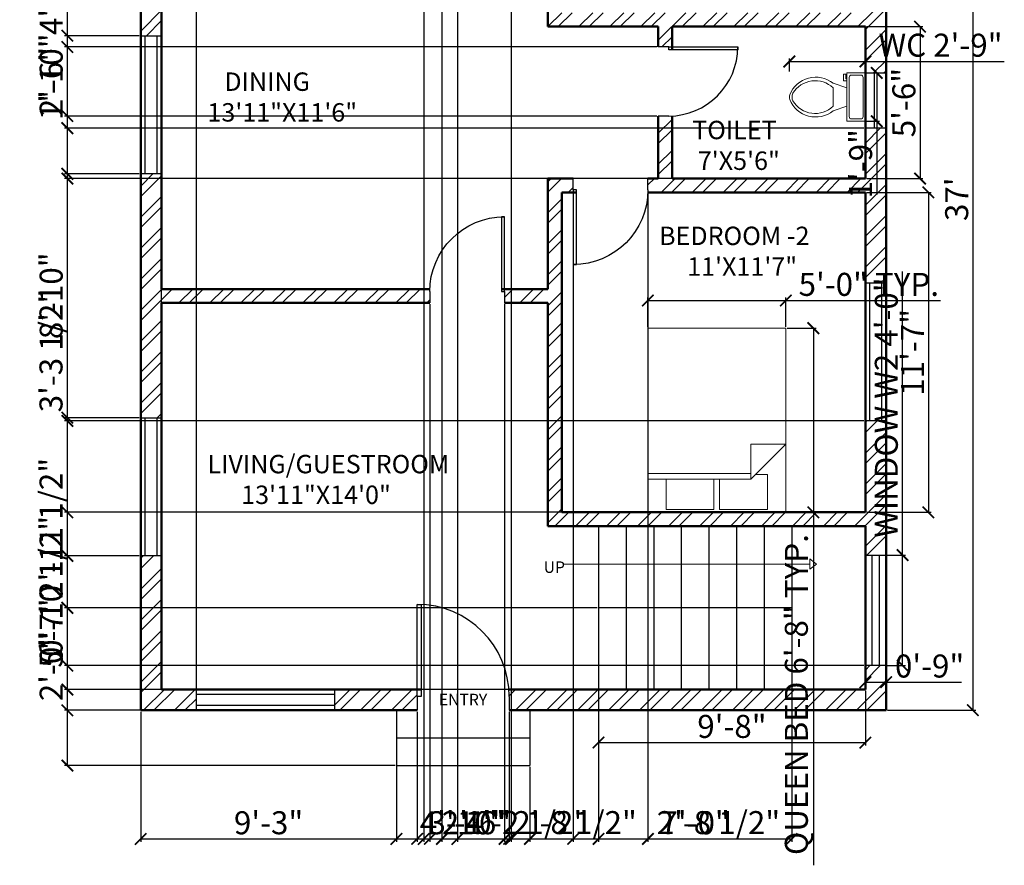
# Model space of a CAD drawing. Units: inches. Extents: x 9 to 670, y -4 to 628.
# Tile 1 of 2: x 9 to 437, y -4 to 363. Entities that reach past the tile are written whole.
import ezdxf

# ---------------------------------------------------------------- set-up
doc = ezdxf.new("R2010")
doc.units = ezdxf.units.IN
for name, color, linetype, lineweight in [('A-ANNO-SYMB', 1, 'Continuous', 18), ('A-AREA-IDEN', 1, 'Continuous', 25), ('A-FLOR-FIXT', 2, 'Continuous', 18), ('A-FLOR-STRS', 7, 'Continuous', 25), ('A-FURN', 2, 'Continuous', 18), ('A-WALL-PATT', 9, 'Continuous', 13), ('DIM', 3, 'Continuous', 18), ('DOORS', 4, 'Continuous', 25), ('TEXT', 1, 'Continuous', 25), ('VENTILATOR', 11, 'Continuous', 25), ('WALLS', 6, 'Continuous', 50), ('WINDOWS', 20, 'Continuous', 25)]:
    doc.layers.add(name, color=color, linetype=linetype, lineweight=lineweight)
doc.styles.get("Standard").update_dxf_attribs({"font": 'arial.ttf'})
doc.dimstyles.new('ISO-25', dxfattribs={"dimtxt": 10, "dimasz": 5, "dimexe": 1.25, "dimexo": 0.625, "dimtad": 1, "dimlunit": 4, "dimtxsty": 'Standard', "dimblk": 'ARCHTICK', "dimcen": 2.5, "dimadec": 0, "dimazin": 0, "dimtfac": 1, "dimtmove": 0, "dimatfit": 3, "dimfxl": 1, "dimarcsym": 0})

# ---------------------------------------------------------------- blocks, each defined once
blk = doc.blocks.new('Toilet - top')
for p, q in [((9.5, -6), (9.5, -2)), ((-10, -8.5), (-8, -8.5)), ((-10, -9.5), (-10, -8.5)), ((-8, -8.5), (-8, -8)), ((-7, -8), (-7, -9.5)), ((-4, -8), (-6, -14)), ((4, -8), (6, -14)), ((-7, -9.5), (-10, -9.5)), ((4, -14), (-4, -14))]:
    blk.add_line(p, q)
blk.add_lwpolyline([(10.5, -8), (10.5, 0), (-10.5, 0), (-10.5, -8)], close=True)
for points in [[(-9.5, -2), (-9.5, -6)], [(8.5, -1), (-8.5, -1)], [(-8.5, -7), (8.5, -7)]]:
    blk.add_lwpolyline(points)
for centre, radius, start, end in [((-8.62, -1.88), 0.884, 81.8699, 188.1301), ((8.62, -1.88), 0.884, 351.8699, 98.1301), ((-8.62, -6.12), 0.884, 171.8699, 278.1301), ((8.62, -6.12), 0.884, 261.8699, 8.1301), ((3.52, -21.58), 12.17, 141.4691, 247.9714), ((4.2, -21.82), 11.33, 136.3677, 238.9468), ((-3.52, -21.58), 12.17, 292.0284, 38.5307), ((-4.2, -21.82), 11.33, 301.053, 43.6321), ((0, -27.88), 4, 245.7318, 294.2682), ((0, -29), 4, 254.8605, 285.1395)]:
    blk.add_arc(centre, radius, start, end)
blk = doc.blocks.new('Bed - Queen')
for p, q in [((0, -80.00003), (0, 0)), ((0, 0), (59.99999, 0)), ((59.99999, 0), (59.99999, -80.00003)), ((7.99999, -1.2), (28.79998, -1.2)), ((7.99999, -14.4), (7.99999, -1.2)), ((28.79998, -1.2), (28.79998, -14.4)), ((31.19999, -1.2), (51.99999, -1.2)), ((31.19999, -14.4), (31.19999, -1.2)), ((51.99999, -1.2), (51.99999, -16.4)), ((0, -14.4), (44.8, -14.4)), ((44.8, -16.8), (0, -16.8)), ((59.99999, -29.6), (44.8, -14.4)), ((44.8, -14.4), (44.8, -29.6)), ((51.99999, -16.4), (46.79936, -16.4)), ((44.8, -29.6), (59.99999, -29.6)), ((59.99999, -80.00003), (0, -80.00003))]:
    blk.add_line(p, q)
blk = doc.blocks.new('*U8')
for p, q in [((0, 0), (0, -6)), ((40, 0), (40, -6))]:
    blk.add_line(p, q)
blk.add_lwpolyline([(0, 0), (0, 40), (1.75, 40), (1.75, 0)], close=True)
blk.add_arc((0, 0), 40, 0, 90)
blk = doc.blocks.new('W2')
at = {"layer": 'WINDOWS'}
for p, q in [((1126.75, 2245.25), (1135.75, 2245.25)), ((1126.75, 2197.25), (1126.75, 2245.25)), ((1129.75, 2197.25), (1129.75, 2245.25)), ((1132.75, 2245.25), (1132.75, 2197.25)), ((1135.75, 2245.25), (1135.75, 2197.25)), ((1135.75, 2197.25), (1126.75, 2197.25))]:
    blk.add_line(p, q, dxfattribs=at)
blk = doc.blocks.new('W1')
at = {"layer": 'WINDOWS'}
for p, q in [((1078.63, 2170.04), (1087.63, 2170.04)), ((1078.63, 2110.04), (1078.63, 2170.04)), ((1080.63, 2110.04), (1080.63, 2170.04)), ((1085.63, 2170.04), (1085.63, 2110.04)), ((1087.63, 2170.04), (1087.63, 2110.04)), ((1087.63, 2110.04), (1078.63, 2110.04))]:
    blk.add_line(p, q, dxfattribs=at)
blk = doc.blocks.new('VENTILATOR')
at = {"layer": 'VENTILATOR'}
for p, q in [((1084.96, 2166.43), (1093.96, 2166.43)), ((1084.96, 2142.43), (1084.96, 2166.43)), ((1088.96, 2142.43), (1088.96, 2166.43)), ((1089.96, 2166.43), (1089.96, 2142.43)), ((1093.96, 2166.43), (1093.96, 2142.43)), ((1093.96, 2142.43), (1084.96, 2142.43))]:
    blk.add_line(p, q, dxfattribs=at)
blk = doc.blocks.new('_ArchTick')
at = {"color": 0, "linetype": 'ByBlock', "const_width": 0.15}
blk.add_lwpolyline([(-0.5, -0.5), (0.5, 0.5)], dxfattribs=at)
blk = doc.blocks.new('*D13')
at = {"layer": 'Defpoints', "color": 0, "transparency": 16777216}
for p in [(376.85, 360.12), (376.85, 294.12), (400.61, 294.12)]:
    blk.add_point(p, dxfattribs=at)
at = {"layer": 'DIM', "color": 0, "lineweight": -2, "transparency": 16777216}
for p, q in [((377.48, 360.12), (401.86, 360.12)), ((400.61, 360.12), (400.61, 294.12)), ((377.48, 294.12), (401.86, 294.12))]:
    blk.add_line(p, q, dxfattribs=at)
at = {"layer": 'DIM', "color": 0, "lineweight": -2, "transparency": 16777216, "xscale": 5, "yscale": 5, "zscale": 5}
for p, rotation in [((400.61, 360.12), 90), ((400.61, 294.12), 270)]:
    blk.add_blockref('_ArchTick', p, dxfattribs=dict(at, rotation=rotation))
at = {"layer": 'DIM', "color": 0, "transparency": 16777216, "insert": (394.88, 327.12), "char_height": 10, "attachment_point": 5, "rotation": 90}
blk.add_mtext('5\'-6"', dxfattribs=at)
blk = doc.blocks.new('*D14')
at = {"layer": 'Defpoints', "color": 0, "transparency": 16777216}
for p in [(376.85, 288.12), (376.85, 149.12), (404.24, 149.12)]:
    blk.add_point(p, dxfattribs=at)
at = {"layer": 'DIM', "color": 0, "lineweight": -2, "transparency": 16777216}
for p, q in [((377.48, 288.12), (405.49, 288.12)), ((404.24, 288.12), (404.24, 149.12)), ((377.48, 149.12), (405.49, 149.12))]:
    blk.add_line(p, q, dxfattribs=at)
at = {"layer": 'DIM', "color": 0, "lineweight": -2, "transparency": 16777216, "xscale": 5, "yscale": 5, "zscale": 5}
for p, rotation in [((404.24, 288.12), 90), ((404.24, 149.12), 270)]:
    blk.add_blockref('_ArchTick', p, dxfattribs=dict(at, rotation=rotation))
at = {"layer": 'DIM', "color": 0, "transparency": 16777216, "insert": (398.59, 218.62), "char_height": 10, "attachment_point": 5, "rotation": 90}
blk.add_mtext('11\'-7"', dxfattribs=at)
blk = doc.blocks.new('*D15')
at = {"layer": 'Defpoints', "color": 0, "transparency": 16777216}
for p in [(385.85, 507.12), (385.85, 63.12), (423.57, 63.12)]:
    blk.add_point(p, dxfattribs=at)
at = {"layer": 'DIM', "color": 0, "lineweight": -2, "transparency": 16777216}
for p, q in [((386.48, 507.12), (424.82, 507.12)), ((423.57, 507.12), (423.57, 63.12)), ((386.48, 63.12), (424.82, 63.12))]:
    blk.add_line(p, q, dxfattribs=at)
at = {"layer": 'DIM', "color": 0, "lineweight": -2, "transparency": 16777216, "xscale": 5, "yscale": 5, "zscale": 5}
for p, rotation in [((423.57, 507.12), 90), ((423.57, 63.12), 270)]:
    blk.add_blockref('_ArchTick', p, dxfattribs=dict(at, rotation=rotation))
at = {"layer": 'DIM', "color": 0, "transparency": 16777216, "insert": (417.84, 285.12), "char_height": 10, "attachment_point": 5, "rotation": 90}
blk.add_mtext("37'", dxfattribs=at)
blk = doc.blocks.new('*D20')
at = {"layer": 'Defpoints', "color": 0, "transparency": 16777216}
for p in [(260.85, 72.12), (376.85, 72.12), (376.85, 49.08)]:
    blk.add_point(p, dxfattribs=at)
at = {"layer": 'DIM', "color": 0, "lineweight": -2, "transparency": 16777216}
for p, q in [((260.85, 71.49), (260.85, 47.83)), ((376.85, 71.49), (376.85, 47.83)), ((260.85, 49.08), (376.85, 49.08))]:
    blk.add_line(p, q, dxfattribs=at)
at = {"layer": 'DIM', "color": 0, "lineweight": -2, "transparency": 16777216, "xscale": 5, "yscale": 5, "zscale": 5, "rotation": 180}
blk.add_blockref('_ArchTick', (260.85, 49.08), dxfattribs=at)
at = {"layer": 'DIM', "color": 0, "lineweight": -2, "transparency": 16777216, "xscale": 5, "yscale": 5, "zscale": 5}
blk.add_blockref('_ArchTick', (376.85, 49.08), dxfattribs=at)
at = {"layer": 'DIM', "color": 0, "transparency": 16777216, "insert": (318.85, 54.81), "char_height": 10, "attachment_point": 5}
blk.add_mtext('9\'-8"', dxfattribs=at)
blk = doc.blocks.new('*D23')
at = {"layer": 'Defpoints', "color": 0, "transparency": 16777216}
for p in [(385.85, 130.51), (393.05, 130.51), (385.85, 82.51)]:
    blk.add_point(p, dxfattribs=at)
at = {"layer": 'DIM', "color": 0, "lineweight": -2, "transparency": 16777216}
for p, q in [((393.05, 130.51), (393.05, 253.77)), ((386.48, 130.51), (394.3, 130.51)), ((393.05, 82.51), (393.05, 130.51)), ((386.48, 82.51), (394.3, 82.51))]:
    blk.add_line(p, q, dxfattribs=at)
at = {"layer": 'DIM', "color": 0, "lineweight": -2, "transparency": 16777216, "xscale": 5, "yscale": 5, "zscale": 5}
for p, rotation in [((393.05, 130.51), 90), ((393.05, 82.51), 270)]:
    blk.add_blockref('_ArchTick', p, dxfattribs=dict(at, rotation=rotation))
at = {"layer": 'DIM', "color": 0, "transparency": 16777216, "insert": (387.25, 194.64), "char_height": 10, "attachment_point": 5, "rotation": 90}
blk.add_mtext('WINDOW W2 4\'-0"', dxfattribs=at)
blk = doc.blocks.new('*D24')
at = {"layer": 'Defpoints', "color": 0, "transparency": 16777216}
for p in [(376.85, 82.51), (385.85, 82.51), (385.85, 75.31)]:
    blk.add_point(p, dxfattribs=at)
at = {"layer": 'DIM', "color": 0, "lineweight": -2, "transparency": 16777216}
for p, q in [((376.85, 81.89), (376.85, 74.06)), ((385.85, 81.89), (385.85, 74.06)), ((376.85, 75.31), (385.85, 75.31)), ((385.85, 75.31), (418.68, 75.31))]:
    blk.add_line(p, q, dxfattribs=at)
at = {"layer": 'DIM', "color": 0, "lineweight": -2, "transparency": 16777216, "xscale": 5, "yscale": 5, "zscale": 5, "rotation": 180}
blk.add_blockref('_ArchTick', (376.85, 75.31), dxfattribs=at)
at = {"layer": 'DIM', "color": 0, "lineweight": -2, "transparency": 16777216, "xscale": 5, "yscale": 5, "zscale": 5}
blk.add_blockref('_ArchTick', (385.85, 75.31), dxfattribs=at)
at = {"layer": 'DIM', "color": 0, "transparency": 16777216, "insert": (404.77, 81.04), "char_height": 10, "attachment_point": 5}
blk.add_mtext('0\'-9"', dxfattribs=at)
blk = doc.blocks.new('*D27')
at = {"layer": 'Defpoints', "color": 0, "transparency": 16777216}
for p in [(376.85, 344.96), (343.8, 340), (376.85, 340)]:
    blk.add_point(p, dxfattribs=at)
at = {"layer": 'DIM', "color": 0, "lineweight": -2, "transparency": 16777216}
for p, q in [((343.8, 340.63), (343.8, 346.21)), ((343.8, 344.96), (376.85, 344.96)), ((376.85, 340.63), (376.85, 346.21)), ((376.85, 344.96), (437.25, 344.96))]:
    blk.add_line(p, q, dxfattribs=at)
at = {"layer": 'DIM', "color": 0, "lineweight": -2, "transparency": 16777216, "xscale": 5, "yscale": 5, "zscale": 5, "rotation": 180}
blk.add_blockref('_ArchTick', (343.8, 344.96), dxfattribs=at)
at = {"layer": 'DIM', "color": 0, "lineweight": -2, "transparency": 16777216, "xscale": 5, "yscale": 5, "zscale": 5}
blk.add_blockref('_ArchTick', (376.85, 344.96), dxfattribs=at)
at = {"layer": 'DIM', "color": 0, "transparency": 16777216, "insert": (409.55, 350.75), "char_height": 10, "attachment_point": 5}
blk.add_mtext('WC 2\'-9"', dxfattribs=at)
blk = doc.blocks.new('*D28')
at = {"layer": 'Defpoints', "color": 0, "transparency": 16777216}
for p in [(376.85, 340), (376.85, 319), (381.81, 319)]:
    blk.add_point(p, dxfattribs=at)
at = {"layer": 'DIM', "color": 0, "lineweight": -2, "transparency": 16777216}
for p, q in [((377.48, 340), (383.06, 340)), ((381.81, 340), (381.81, 319)), ((377.48, 319), (383.06, 319)), ((381.81, 319), (381.81, 287.11))]:
    blk.add_line(p, q, dxfattribs=at)
at = {"layer": 'DIM', "color": 0, "lineweight": -2, "transparency": 16777216, "xscale": 5, "yscale": 5, "zscale": 5}
for p, rotation in [((381.81, 340), 90), ((381.81, 319), 270)]:
    blk.add_blockref('_ArchTick', p, dxfattribs=dict(at, rotation=rotation))
at = {"layer": 'DIM', "color": 0, "transparency": 16777216, "insert": (376.08, 300.55), "char_height": 10, "attachment_point": 5, "rotation": 90}
blk.add_mtext('1\'-9"', dxfattribs=at)
blk = doc.blocks.new('*D29')
at = {"layer": 'Defpoints', "color": 0, "transparency": 16777216}
for p in [(342.24, 229.12), (342.24, 149.12), (354.24, 149.12)]:
    blk.add_point(p, dxfattribs=at)
at = {"layer": 'DIM', "color": 0, "lineweight": -2, "transparency": 16777216}
for p, q in [((342.87, 229.12), (355.49, 229.12)), ((354.24, 229.12), (354.24, 149.12)), ((342.87, 149.12), (355.49, 149.12)), ((354.24, 149.12), (354.24, -4.23))]:
    blk.add_line(p, q, dxfattribs=at)
at = {"layer": 'DIM', "color": 0, "lineweight": -2, "transparency": 16777216, "xscale": 5, "yscale": 5, "zscale": 5}
for p, rotation in [((354.24, 229.12), 90), ((354.24, 149.12), 270)]:
    blk.add_blockref('_ArchTick', p, dxfattribs=dict(at, rotation=rotation))
at = {"layer": 'DIM', "color": 0, "transparency": 16777216, "insert": (348.14, 69.94), "char_height": 10, "attachment_point": 5, "rotation": 90}
blk.add_mtext('QUEEN BED 6\'-8" TYP.', dxfattribs=at)
blk = doc.blocks.new('*D30')
at = {"layer": 'Defpoints', "color": 0, "transparency": 16777216}
for p in [(342.24, 241.12), (282.24, 229.12), (342.24, 229.12)]:
    blk.add_point(p, dxfattribs=at)
at = {"layer": 'DIM', "color": 0, "lineweight": -2, "transparency": 16777216}
for p, q in [((282.24, 229.74), (282.24, 242.37)), ((282.24, 241.12), (342.24, 241.12)), ((342.24, 229.74), (342.24, 242.37)), ((342.24, 241.12), (409.45, 241.12))]:
    blk.add_line(p, q, dxfattribs=at)
at = {"layer": 'DIM', "color": 0, "lineweight": -2, "transparency": 16777216, "xscale": 5, "yscale": 5, "zscale": 5, "rotation": 180}
blk.add_blockref('_ArchTick', (282.24, 241.12), dxfattribs=at)
at = {"layer": 'DIM', "color": 0, "lineweight": -2, "transparency": 16777216, "xscale": 5, "yscale": 5, "zscale": 5}
blk.add_blockref('_ArchTick', (342.24, 241.12), dxfattribs=at)
at = {"layer": 'DIM', "color": 0, "transparency": 16777216, "insert": (378.35, 246.85), "char_height": 10, "attachment_point": 5}
blk.add_mtext('5\'-0" TYP.', dxfattribs=at)
blk = doc.blocks.new('*D35')
at = {"layer": 'Defpoints', "color": 0, "transparency": 16777216}
for p in [(173.01, 39.12), (231.01, 39.12), (231.01, 7.22)]:
    blk.add_point(p, dxfattribs=at)
at = {"layer": 'DIM', "color": 0, "lineweight": -2, "transparency": 16777216}
for p, q in [((173.01, 38.49), (173.01, 5.97)), ((231.01, 38.49), (231.01, 5.97)), ((173.01, 7.22), (231.01, 7.22))]:
    blk.add_line(p, q, dxfattribs=at)
at = {"layer": 'DIM', "color": 0, "lineweight": -2, "transparency": 16777216, "xscale": 5, "yscale": 5, "zscale": 5, "rotation": 180}
blk.add_blockref('_ArchTick', (173.01, 7.22), dxfattribs=at)
at = {"layer": 'DIM', "color": 0, "lineweight": -2, "transparency": 16777216, "xscale": 5, "yscale": 5, "zscale": 5}
blk.add_blockref('_ArchTick', (231.01, 7.22), dxfattribs=at)
at = {"layer": 'DIM', "color": 0, "transparency": 16777216, "insert": (202.01, 12.95), "char_height": 10, "attachment_point": 5}
blk.add_mtext('4\'-10"', dxfattribs=at)
blk = doc.blocks.new('*D36')
at = {"layer": 'Defpoints', "color": 0, "transparency": 16777216}
for p in [(29.95, 63.12), (173.01, 63.12), (173.01, 39.12)]:
    blk.add_point(p, dxfattribs=at)
at = {"layer": 'DIM', "color": 0, "lineweight": -2, "transparency": 16777216}
for p, q in [((29.95, 63.12), (29.95, 96.12)), ((172.39, 63.12), (28.7, 63.12)), ((29.95, 39.12), (29.95, 63.12)), ((172.39, 39.12), (28.7, 39.12))]:
    blk.add_line(p, q, dxfattribs=at)
at = {"layer": 'DIM', "color": 0, "lineweight": -2, "transparency": 16777216, "xscale": 5, "yscale": 5, "zscale": 5}
for p, rotation in [((29.95, 63.12), 90), ((29.95, 39.12), 270)]:
    blk.add_blockref('_ArchTick', p, dxfattribs=dict(at, rotation=rotation))
at = {"layer": 'DIM', "color": 0, "transparency": 16777216, "insert": (24.22, 82.12), "char_height": 10, "attachment_point": 5, "rotation": 90}
blk.add_mtext('2\'-0"', dxfattribs=at)
blk = doc.blocks.new('*D37')
at = {"layer": 'Defpoints', "color": 0, "transparency": 16777216}
for p in [(182.01, 63.12), (222.01, 63.12), (222.01, 7.22)]:
    blk.add_point(p, dxfattribs=at)
at = {"layer": 'DIM', "color": 0, "lineweight": -2, "transparency": 16777216}
for p, q in [((182.01, 62.49), (182.01, 5.97)), ((222.01, 62.49), (222.01, 5.97)), ((182.01, 7.22), (222.01, 7.22))]:
    blk.add_line(p, q, dxfattribs=at)
at = {"layer": 'DIM', "color": 0, "lineweight": -2, "transparency": 16777216, "xscale": 5, "yscale": 5, "zscale": 5, "rotation": 180}
blk.add_blockref('_ArchTick', (182.01, 7.22), dxfattribs=at)
at = {"layer": 'DIM', "color": 0, "lineweight": -2, "transparency": 16777216, "xscale": 5, "yscale": 5, "zscale": 5}
blk.add_blockref('_ArchTick', (222.01, 7.22), dxfattribs=at)
at = {"layer": 'DIM', "color": 0, "transparency": 16777216, "insert": (202.01, 12.95), "char_height": 10, "attachment_point": 5}
blk.add_mtext('3\'-4"', dxfattribs=at)
blk = doc.blocks.new('*D38')
at = {"layer": 'Defpoints', "color": 0, "transparency": 16777216}
for p in [(61.85, 63.12), (173.01, 63.12), (173.01, 7.22)]:
    blk.add_point(p, dxfattribs=at)
at = {"layer": 'DIM', "color": 0, "lineweight": -2, "transparency": 16777216}
for p, q in [((61.85, 62.49), (61.85, 5.97)), ((173.01, 62.49), (173.01, 5.97)), ((61.85, 7.22), (173.01, 7.22))]:
    blk.add_line(p, q, dxfattribs=at)
at = {"layer": 'DIM', "color": 0, "lineweight": -2, "transparency": 16777216, "xscale": 5, "yscale": 5, "zscale": 5, "rotation": 180}
blk.add_blockref('_ArchTick', (61.85, 7.22), dxfattribs=at)
at = {"layer": 'DIM', "color": 0, "lineweight": -2, "transparency": 16777216, "xscale": 5, "yscale": 5, "zscale": 5}
blk.add_blockref('_ArchTick', (173.01, 7.22), dxfattribs=at)
at = {"layer": 'DIM', "color": 0, "transparency": 16777216, "insert": (117.43, 12.95), "char_height": 10, "attachment_point": 5}
blk.add_mtext('9\'-3"', dxfattribs=at)
blk = doc.blocks.new('*D39')
at = {"layer": 'Defpoints', "color": 0, "transparency": 16777216}
for p in [(187.51, 240.12), (220.03, 240.12), (220.03, 7.22)]:
    blk.add_point(p, dxfattribs=at)
at = {"layer": 'DIM', "color": 0, "lineweight": -2, "transparency": 16777216}
for p, q in [((187.51, 239.49), (187.51, 5.97)), ((220.03, 239.49), (220.03, 5.97)), ((187.51, 7.22), (220.03, 7.22)), ((220.03, 7.22), (276.34, 7.22))]:
    blk.add_line(p, q, dxfattribs=at)
at = {"layer": 'DIM', "color": 0, "lineweight": -2, "transparency": 16777216, "xscale": 5, "yscale": 5, "zscale": 5, "rotation": 180}
blk.add_blockref('_ArchTick', (187.51, 7.22), dxfattribs=at)
at = {"layer": 'DIM', "color": 0, "lineweight": -2, "transparency": 16777216, "xscale": 5, "yscale": 5, "zscale": 5}
blk.add_blockref('_ArchTick', (220.03, 7.22), dxfattribs=at)
at = {"layer": 'DIM', "color": 0, "transparency": 16777216, "insert": (250.68, 13.01), "char_height": 10, "attachment_point": 5}
blk.add_mtext('2\'-8 1/2"', dxfattribs=at)
blk = doc.blocks.new('*D40')
at = {"layer": 'Defpoints', "color": 0, "transparency": 16777216}
for p in [(249.83, 289.24), (282.33, 288.12), (282.33, 7.22)]:
    blk.add_point(p, dxfattribs=at)
at = {"layer": 'DIM', "color": 0, "lineweight": -2, "transparency": 16777216}
for p, q in [((249.83, 288.62), (249.83, 5.97)), ((282.33, 287.49), (282.33, 5.97)), ((249.83, 7.22), (282.33, 7.22)), ((282.33, 7.22), (338.63, 7.22))]:
    blk.add_line(p, q, dxfattribs=at)
at = {"layer": 'DIM', "color": 0, "lineweight": -2, "transparency": 16777216, "xscale": 5, "yscale": 5, "zscale": 5, "rotation": 180}
blk.add_blockref('_ArchTick', (249.83, 7.22), dxfattribs=at)
at = {"layer": 'DIM', "color": 0, "lineweight": -2, "transparency": 16777216, "xscale": 5, "yscale": 5, "zscale": 5}
blk.add_blockref('_ArchTick', (282.33, 7.22), dxfattribs=at)
at = {"layer": 'DIM', "color": 0, "transparency": 16777216, "insert": (312.98, 13.01), "char_height": 10, "attachment_point": 5}
blk.add_mtext('2\'-8 1/2"', dxfattribs=at)
blk = doc.blocks.new('*D41')
at = {"layer": 'Defpoints', "color": 0, "transparency": 16777216}
for p in [(29.95, 351.29), (286.85, 351.29), (286.85, 321.26)]:
    blk.add_point(p, dxfattribs=at)
at = {"layer": 'DIM', "color": 0, "lineweight": -2, "transparency": 16777216}
for p, q in [((286.23, 351.29), (28.7, 351.29)), ((29.95, 321.26), (29.95, 351.29)), ((286.23, 321.26), (28.7, 321.26))]:
    blk.add_line(p, q, dxfattribs=at)
at = {"layer": 'DIM', "color": 0, "lineweight": -2, "transparency": 16777216, "xscale": 5, "yscale": 5, "zscale": 5}
for p, rotation in [((29.95, 351.29), 90), ((29.95, 321.26), 270)]:
    blk.add_blockref('_ArchTick', p, dxfattribs=dict(at, rotation=rotation))
at = {"layer": 'DIM', "color": 0, "transparency": 16777216, "insert": (24.22, 336.28), "char_height": 10, "attachment_point": 5, "rotation": 90}
blk.add_mtext('2\'-6"', dxfattribs=at)
blk = doc.blocks.new('*D43')
at = {"layer": 'Defpoints', "color": 0, "transparency": 16777216}
for p in [(192.78, 413.12), (222.81, 413.12), (222.81, 7.22)]:
    blk.add_point(p, dxfattribs=at)
at = {"layer": 'DIM', "color": 0, "lineweight": -2, "transparency": 16777216}
for p, q in [((192.78, 412.49), (192.78, 5.97)), ((222.81, 412.49), (222.81, 5.97)), ((192.78, 7.22), (222.81, 7.22))]:
    blk.add_line(p, q, dxfattribs=at)
at = {"layer": 'DIM', "color": 0, "lineweight": -2, "transparency": 16777216, "xscale": 5, "yscale": 5, "zscale": 5, "rotation": 180}
blk.add_blockref('_ArchTick', (192.78, 7.22), dxfattribs=at)
at = {"layer": 'DIM', "color": 0, "lineweight": -2, "transparency": 16777216, "xscale": 5, "yscale": 5, "zscale": 5}
blk.add_blockref('_ArchTick', (222.81, 7.22), dxfattribs=at)
at = {"layer": 'DIM', "color": 0, "transparency": 16777216, "insert": (207.8, 12.95), "char_height": 10, "attachment_point": 5}
blk.add_mtext('2\'-6"', dxfattribs=at)
blk = doc.blocks.new('*D44')
at = {"layer": 'Defpoints', "color": 0, "transparency": 16777216}
for p in [(29.95, 130.21), (61.85, 130.21), (61.85, 63.12)]:
    blk.add_point(p, dxfattribs=at)
at = {"layer": 'DIM', "color": 0, "lineweight": -2, "transparency": 16777216}
for p, q in [((61.23, 130.21), (28.7, 130.21)), ((29.95, 63.12), (29.95, 130.21)), ((61.23, 63.12), (28.7, 63.12))]:
    blk.add_line(p, q, dxfattribs=at)
at = {"layer": 'DIM', "color": 0, "lineweight": -2, "transparency": 16777216, "xscale": 5, "yscale": 5, "zscale": 5}
for p, rotation in [((29.95, 130.21), 90), ((29.95, 63.12), 270)]:
    blk.add_blockref('_ArchTick', p, dxfattribs=dict(at, rotation=rotation))
at = {"layer": 'DIM', "color": 0, "transparency": 16777216, "insert": (24.24, 96.67), "char_height": 10, "attachment_point": 5, "rotation": 90}
blk.add_mtext('5\'-7"', dxfattribs=at)
blk = doc.blocks.new('*D45')
at = {"layer": 'Defpoints', "color": 0, "transparency": 16777216}
for p in [(29.95, 296.16), (61.85, 296.16), (61.85, 190.21)]:
    blk.add_point(p, dxfattribs=at)
at = {"layer": 'DIM', "color": 0, "lineweight": -2, "transparency": 16777216}
for p, q in [((61.23, 296.16), (28.7, 296.16)), ((29.95, 190.21), (29.95, 296.16)), ((61.23, 190.21), (28.7, 190.21))]:
    blk.add_line(p, q, dxfattribs=at)
at = {"layer": 'DIM', "color": 0, "lineweight": -2, "transparency": 16777216, "xscale": 5, "yscale": 5, "zscale": 5}
for p, rotation in [((29.95, 296.16), 90), ((29.95, 190.21), 270)]:
    blk.add_blockref('_ArchTick', p, dxfattribs=dict(at, rotation=rotation))
at = {"layer": 'DIM', "color": 0, "transparency": 16777216, "insert": (24.22, 243.19), "char_height": 10, "attachment_point": 5, "rotation": 90}
blk.add_mtext('8\'-10"', dxfattribs=at)
blk = doc.blocks.new('*D46')
at = {"layer": 'Defpoints', "color": 0, "transparency": 16777216}
for p in [(29.95, 410.46), (61.85, 410.46), (61.85, 356.16)]:
    blk.add_point(p, dxfattribs=at)
at = {"layer": 'DIM', "color": 0, "lineweight": -2, "transparency": 16777216}
for p, q in [((61.23, 410.46), (28.7, 410.46)), ((29.95, 356.16), (29.95, 410.46)), ((61.23, 356.16), (28.7, 356.16))]:
    blk.add_line(p, q, dxfattribs=at)
at = {"layer": 'DIM', "color": 0, "lineweight": -2, "transparency": 16777216, "xscale": 5, "yscale": 5, "zscale": 5}
for p, rotation in [((29.95, 410.46), 90), ((29.95, 356.16), 270)]:
    blk.add_blockref('_ArchTick', p, dxfattribs=dict(at, rotation=rotation))
at = {"layer": 'DIM', "color": 0, "transparency": 16777216, "insert": (24.16, 383.31), "char_height": 10, "attachment_point": 5, "rotation": 90}
blk.add_mtext('4\'-6 1/2"', dxfattribs=at)
blk = doc.blocks.new('*D47')
at = {"layer": 'Defpoints', "color": 0, "transparency": 16777216}
for p in [(86.08, 539.02), (70.85, 72.12), (86.08, 72.12)]:
    blk.add_point(p, dxfattribs=at)
at = {"layer": 'DIM', "color": 0, "lineweight": -2, "transparency": 16777216}
for p, q in [((70.85, 72.74), (70.85, 540.27)), ((86.08, 72.74), (86.08, 540.27)), ((70.85, 539.02), (86.08, 539.02)), ((86.08, 539.02), (117.98, 539.02))]:
    blk.add_line(p, q, dxfattribs=at)
at = {"layer": 'DIM', "color": 0, "lineweight": -2, "transparency": 16777216, "xscale": 5, "yscale": 5, "zscale": 5, "rotation": 180}
blk.add_blockref('_ArchTick', (70.85, 539.02), dxfattribs=at)
at = {"layer": 'DIM', "color": 0, "lineweight": -2, "transparency": 16777216, "xscale": 5, "yscale": 5, "zscale": 5}
blk.add_blockref('_ArchTick', (86.08, 539.02), dxfattribs=at)
at = {"layer": 'DIM', "color": 0, "transparency": 16777216, "insert": (104.53, 544.75), "char_height": 10, "attachment_point": 5}
blk.add_mtext('1\'-3"', dxfattribs=at)
blk = doc.blocks.new('*D48')
at = {"layer": 'Defpoints', "color": 0, "transparency": 16777216}
for p in [(184.85, 498.12), (199.5, 498.12), (199.5, 7.22)]:
    blk.add_point(p, dxfattribs=at)
at = {"layer": 'DIM', "color": 0, "lineweight": -2, "transparency": 16777216}
for p, q in [((184.85, 497.49), (184.85, 5.97)), ((199.5, 497.49), (199.5, 5.97)), ((184.85, 7.22), (199.5, 7.22)), ((199.5, 7.22), (254.69, 7.22))]:
    blk.add_line(p, q, dxfattribs=at)
at = {"layer": 'DIM', "color": 0, "lineweight": -2, "transparency": 16777216, "xscale": 5, "yscale": 5, "zscale": 5, "rotation": 180}
blk.add_blockref('_ArchTick', (184.85, 7.22), dxfattribs=at)
at = {"layer": 'DIM', "color": 0, "lineweight": -2, "transparency": 16777216, "xscale": 5, "yscale": 5, "zscale": 5}
blk.add_blockref('_ArchTick', (199.5, 7.22), dxfattribs=at)
at = {"layer": 'DIM', "color": 0, "transparency": 16777216, "insert": (229.6, 13.01), "char_height": 10, "attachment_point": 5}
blk.add_mtext('1\'-2 1/2"', dxfattribs=at)
blk = doc.blocks.new('*D50')
at = {"layer": 'Defpoints', "color": 0, "transparency": 16777216}
for p in [(29.95, 316), (376.85, 316), (376.85, 294.12)]:
    blk.add_point(p, dxfattribs=at)
at = {"layer": 'DIM', "color": 0, "lineweight": -2, "transparency": 16777216}
for p, q in [((29.95, 316), (29.95, 355.66)), ((376.23, 316), (28.7, 316)), ((29.95, 294.12), (29.95, 316)), ((376.23, 294.12), (28.7, 294.12))]:
    blk.add_line(p, q, dxfattribs=at)
at = {"layer": 'DIM', "color": 0, "lineweight": -2, "transparency": 16777216, "xscale": 5, "yscale": 5, "zscale": 5}
for p, rotation in [((29.95, 316), 90), ((29.95, 294.12), 270)]:
    blk.add_blockref('_ArchTick', p, dxfattribs=dict(at, rotation=rotation))
at = {"layer": 'DIM', "color": 0, "transparency": 16777216, "insert": (24.22, 338.33), "char_height": 10, "attachment_point": 5, "rotation": 90}
blk.add_mtext('1\'-10"', dxfattribs=at)
blk = doc.blocks.new('*D51')
at = {"layer": 'Defpoints', "color": 0, "transparency": 16777216}
for p in [(29.95, 188.84), (376.85, 188.84), (376.85, 149.12)]:
    blk.add_point(p, dxfattribs=at)
at = {"layer": 'DIM', "color": 0, "lineweight": -2, "transparency": 16777216}
for p, q in [((29.95, 188.84), (29.95, 244.96)), ((376.23, 188.84), (28.7, 188.84)), ((29.95, 149.12), (29.95, 188.84)), ((376.23, 149.12), (28.7, 149.12))]:
    blk.add_line(p, q, dxfattribs=at)
at = {"layer": 'DIM', "color": 0, "lineweight": -2, "transparency": 16777216, "xscale": 5, "yscale": 5, "zscale": 5}
for p, rotation in [((29.95, 188.84), 90), ((29.95, 149.12), 270)]:
    blk.add_blockref('_ArchTick', p, dxfattribs=dict(at, rotation=rotation))
at = {"layer": 'DIM', "color": 0, "transparency": 16777216, "insert": (24.15, 219.4), "char_height": 10, "attachment_point": 5, "rotation": 90}
blk.add_mtext('3\'-3 1/2"', dxfattribs=at)
blk = doc.blocks.new('*D52')
at = {"layer": 'Defpoints', "color": 0, "transparency": 16777216}
for p in [(29.95, 82.51), (376.85, 82.51), (376.85, 72.12)]:
    blk.add_point(p, dxfattribs=at)
at = {"layer": 'DIM', "color": 0, "lineweight": -2, "transparency": 16777216}
for p, q in [((29.95, 82.51), (29.95, 146.41)), ((376.23, 82.51), (28.7, 82.51)), ((29.95, 72.12), (29.95, 82.51)), ((376.23, 72.12), (28.7, 72.12))]:
    blk.add_line(p, q, dxfattribs=at)
at = {"layer": 'DIM', "color": 0, "lineweight": -2, "transparency": 16777216, "xscale": 5, "yscale": 5, "zscale": 5}
for p, rotation in [((29.95, 82.51), 90), ((29.95, 72.12), 270)]:
    blk.add_blockref('_ArchTick', p, dxfattribs=dict(at, rotation=rotation))
at = {"layer": 'DIM', "color": 0, "transparency": 16777216, "insert": (24.16, 116.96), "char_height": 10, "attachment_point": 5, "rotation": 90}
blk.add_mtext('0\'-10 1/2"', dxfattribs=at)
blk = doc.blocks.new('*D53')
at = {"layer": 'Defpoints', "color": 0, "transparency": 16777216}
for p in [(260.85, 72.12), (344.85, 72.12), (344.85, 7.22)]:
    blk.add_point(p, dxfattribs=at)
at = {"layer": 'DIM', "color": 0, "lineweight": -2, "transparency": 16777216}
for p, q in [((260.85, 71.49), (260.85, 5.97)), ((344.85, 71.49), (344.85, 5.97)), ((260.85, 7.22), (344.85, 7.22))]:
    blk.add_line(p, q, dxfattribs=at)
at = {"layer": 'DIM', "color": 0, "lineweight": -2, "transparency": 16777216, "xscale": 5, "yscale": 5, "zscale": 5, "rotation": 180}
blk.add_blockref('_ArchTick', (260.85, 7.22), dxfattribs=at)
at = {"layer": 'DIM', "color": 0, "lineweight": -2, "transparency": 16777216, "xscale": 5, "yscale": 5, "zscale": 5}
blk.add_blockref('_ArchTick', (344.85, 7.22), dxfattribs=at)
at = {"layer": 'DIM', "color": 0, "transparency": 16777216, "insert": (302.85, 12.95), "char_height": 10, "attachment_point": 5}
blk.add_mtext('7\'-0"', dxfattribs=at)
blk = doc.blocks.new('*D54')
at = {"layer": 'Defpoints', "color": 0, "transparency": 16777216}
for p in [(29.95, 107.62), (260.85, 107.62), (260.85, 72.12)]:
    blk.add_point(p, dxfattribs=at)
at = {"layer": 'DIM', "color": 0, "lineweight": -2, "transparency": 16777216}
for p, q in [((29.95, 107.62), (29.95, 171.69)), ((260.23, 107.62), (28.7, 107.62)), ((29.95, 72.12), (29.95, 107.62)), ((260.23, 72.12), (28.7, 72.12))]:
    blk.add_line(p, q, dxfattribs=at)
at = {"layer": 'DIM', "color": 0, "lineweight": -2, "transparency": 16777216, "xscale": 5, "yscale": 5, "zscale": 5}
for p, rotation in [((29.95, 107.62), 90), ((29.95, 72.12), 270)]:
    blk.add_blockref('_ArchTick', p, dxfattribs=dict(at, rotation=rotation))
at = {"layer": 'DIM', "color": 0, "transparency": 16777216, "insert": (24.16, 142.16), "char_height": 10, "attachment_point": 5, "rotation": 90}
blk.add_mtext('2\'-11 1/2"', dxfattribs=at)

msp = doc.modelspace()

# ---------------------------------------------------------------- hatches: boundary and pattern name
at = {"layer": 'A-WALL-PATT'}
h = msp.add_hatch(dxfattribs=at)
h.set_pattern_fill('ANSI32', color=256)
h.paths.add_polyline_path([(70.851, 384.119), (124.851, 384.119), (124.851, 390.119), (70.851, 390.119), (70.851, 410.46), (61.851, 410.46), (61.851, 356.162), (70.851, 356.162)])
h.paths.add_polyline_path([(199.501, 507.119), (61.851, 507.119), (61.851, 470.46), (70.851, 470.46), (70.851, 498.119), (178.851, 498.119), (178.851, 384.119), (184.851, 384.119), (184.851, 413.119), (192.784, 413.119), (192.784, 417.623), (192.784, 419.119), (184.851, 419.119), (184.851, 498.119), (199.501, 498.119)])
h.paths.add_polyline_path([(244.851, 498.119), (376.851, 498.119), (376.851, 470.602), (385.851, 470.602), (385.851, 507.119), (223.501, 507.119), (223.501, 498.119), (238.851, 498.119), (238.851, 419.119), (222.776, 419.119, -0.0124579), (222.813, 417.623), (222.813, 413.119), (238.851, 413.119), (238.851, 404.582), (243.729, 404.582, -0.0086282), (244.851, 404.563)])
h.paths.add_polyline_path([(385.851, 410.602), (376.851, 410.602), (376.851, 366.119), (244.851, 366.119), (244.851, 372.063), (243.729, 372.063), (238.851, 372.063), (238.851, 360.119), (286.851, 360.119), (286.851, 351.292), (291.355, 351.292), (292.851, 351.292), (292.851, 360.119), (376.851, 360.119), (376.851, 340), (385.851, 340)])
h.paths.add_polyline_path([(385.851, 188.838), (376.851, 188.838), (376.851, 149.119), (244.851, 149.119), (244.851, 288.119), (249.83, 288.119), (249.83, 289.241), (249.83, 294.119), (238.851, 294.119), (238.851, 246.119), (220.031, 246.119), (220.031, 244.997), (220.031, 240.119), (238.851, 240.119), (238.851, 143.119), (244.851, 143.119), (376.851, 143.119), (376.851, 130.511), (385.851, 130.511)])
h.paths.add_polyline_path([(385.851, 316), (376.851, 316), (376.851, 294.119), (292.851, 294.119), (292.851, 321.301, -0.0124579), (291.355, 321.264), (286.851, 321.264), (286.851, 294.119), (282.349, 294.119), (282.349, 289.241, -0.0086282), (282.33, 288.119), (376.851, 288.119), (376.851, 248.838), (385.851, 248.838)])
h.paths.add_polyline_path([(187.53, 246.119), (70.851, 246.119), (70.851, 296.162), (61.851, 296.162), (61.851, 190.214), (70.851, 190.214), (70.851, 240.119), (187.511, 240.119), (187.511, 244.997, -0.0086282)])
h.paths.add_polyline_path([(385.851, 82.511), (376.851, 82.511), (376.851, 72.119), (221.899, 72.119, -0.0187698), (222.012, 69.119), (222.012, 63.119), (385.851, 63.119)])
h.paths.add_polyline_path([(182.012, 69.119), (182.012, 72.119), (146.085, 72.119), (146.085, 63.119), (182.012, 63.119)])
h.paths.add_polyline_path([(86.085, 72.119), (70.851, 72.119), (70.851, 130.214), (61.851, 130.214), (61.851, 63.119), (86.085, 63.119)])

# ---------------------------------------------------------------- linework, layer by layer
at = {"layer": 'A-ANNO-SYMB'}
for p, q in [((352.64, 128.85), (352.64, 124.396)), ((355.678, 126.61), (352.64, 128.85)), ((245.795, 126.61), (352.64, 126.61)), ((352.64, 124.396), (355.678, 126.61))]:
    msp.add_line(p, q, dxfattribs=at)
at = {"layer": 'A-FLOR-STRS'}
for p, q in [((260.851, 143.119), (260.851, 72.119)), ((272.851, 143.119), (272.851, 72.119)), ((284.851, 143.119), (284.851, 72.119)), ((296.851, 143.119), (296.851, 72.119)), ((308.851, 143.119), (308.851, 72.119)), ((320.851, 143.119), (320.851, 72.119)), ((332.851, 143.119), (332.851, 72.119)), ((344.851, 143.119), (344.851, 72.119)), ((344.851, 107.619), (260.851, 107.619)), ((173.012, 63.119), (173.012, 39.119)), ((231.012, 63.119), (231.012, 39.119)), ((173.012, 51.119), (231.012, 51.119)), ((173.012, 39.119), (231.012, 39.119))]:
    msp.add_line(p, q, dxfattribs=at)
at = {"layer": 'WALLS'}
for p, q in [((61.851, 507.119), (61.851, 63.119)), ((385.851, 507.119), (385.851, 63.119)), ((70.851, 384.119), (70.851, 246.119)), ((238.851, 372.063), (238.851, 360.119)), ((238.851, 360.119), (286.851, 360.119)), ((286.851, 360.119), (286.851, 351.292)), ((292.851, 360.119), (292.851, 349.979)), ((292.851, 360.119), (376.851, 360.119)), ((376.851, 360.119), (376.851, 294.119)), ((286.851, 321.264), (286.851, 294.119)), ((292.851, 321.301), (292.851, 294.119)), ((238.851, 294.119), (249.83, 294.119)), ((238.851, 294.119), (238.851, 246.119)), ((282.349, 294.119), (286.851, 294.119)), ((292.851, 294.119), (376.851, 294.119)), ((244.851, 288.119), (251.253, 288.119)), ((244.851, 288.119), (244.851, 149.119)), ((282.33, 288.119), (376.851, 288.119)), ((376.851, 288.119), (376.851, 149.119)), ((70.851, 246.119), (187.53, 246.119)), ((218.608, 246.119), (238.851, 246.119)), ((70.851, 240.119), (187.511, 240.119)), ((70.851, 240.119), (70.851, 72.119)), ((220.031, 240.119), (238.851, 240.119)), ((238.851, 240.119), (238.851, 143.119)), ((244.851, 149.119), (376.851, 149.119)), ((244.851, 143.119), (238.851, 143.119)), ((244.851, 143.119), (376.851, 143.119)), ((376.851, 143.119), (376.851, 72.119)), ((70.851, 72.119), (183.762, 72.119)), ((221.899, 72.119), (376.851, 72.119)), ((61.851, 63.119), (182.012, 63.119)), ((222.012, 63.119), (385.851, 63.119))]:
    msp.add_line(p, q, dxfattribs=at)

# ---------------------------------------------------------------- block references
at = {"layer": 'A-FLOR-FIXT', "rotation": 270}
msp.add_blockref('Toilet - top', (376.851, 329.5), dxfattribs=at)
at = {"layer": 'A-FURN', "xscale": -1, "rotation": 180}
msp.add_blockref('Bed - Queen', (282.244, 149.119), dxfattribs=at)
at = {"layer": 'DOORS'}
for p, xscale, yscale, zscale, rotation in [((291.355, 351.292), 0.750718739775508, 0.750718739775508, 0.750718739775508, 270), ((249.83, 289.241), -0.812986333406137, 0.812986333406137, 0.812986333406137, 180)]:
    msp.add_blockref('*U8', p, dxfattribs=dict(at, xscale=xscale, yscale=yscale, zscale=zscale, rotation=rotation))
at = {"layer": 'DOORS', "xscale": -0.812986333406137, "yscale": 0.812986333406137, "zscale": 0.812986333406137}
msp.add_blockref('*U8', (220.031, 244.997), dxfattribs=at)
at = {"layer": 'DOORS'}
msp.add_blockref('*U8', (182.012, 69.119), dxfattribs=at)
at = {"layer": 'VENTILATOR', "rotation": 180}
msp.add_blockref('VENTILATOR', (1470.812, 2482.427), dxfattribs=at)
at = {"layer": 'WINDOWS'}
for name, p in [('W1', (-1016.781, -1813.883)), ('W1', (-701.781, -1921.207)), ('W1', (-1016.781, -1979.831)), ('W2', (-749.895, -2114.736))]:
    msp.add_blockref(name, p, dxfattribs=at)
at = {"layer": 'WINDOWS', "rotation": 270}
msp.add_blockref('W1', (-2023.96, 1150.75), dxfattribs=at)

# ---------------------------------------------------------------- texts
at = {"layer": 'A-AREA-IDEN', "char_height": 8, "attachment_point": 1}
for s, width, insert in [('   DINING                          \\P13\'11"X11\'6"', 64.44768, (90.858, 340.204)), (' TOILET    \\P  7\'X5\'6"', 58.62227, (299.134, 319.202)), ('BEDROOM -2    \\P     11\'X11\'7"', 76.76666, (287.182, 273.214)), ('LIVING/GUESTROOM                           \\P      13\'11"X14\'0"', 124.03495, (90.858, 174.061))]:
    msp.add_mtext_dynamic_manual_height_columns(s, width=width, gutter_width=12.5, heights=[0], dxfattribs=dict(at, insert=insert))
at = {"layer": 'TEXT', "char_height": 5, "attachment_point": 1}
for s, width, insert in [('UP', 8.8299, (237.022, 127.796)), ('ENTRY', 21.1951, (191.465, 70.266))]:
    msp.add_mtext_dynamic_manual_height_columns(s, width=width, gutter_width=12.5, heights=[0], dxfattribs=dict(at, insert=insert))

# ---------------------------------------------------------------- dimensions: what is measured, and where the dimension line sits
at = {"layer": 'DIM'}
for base, p1, p2, override, picture, middle in [((86.085, 539.019), (70.851, 72.119), (86.085, 72.119), {"dimdec": 1, "dimlfac": 1, "dimrnd": 0, "dimzin": 1, "dimdsep": 46, "dimlunit": 4, "dimfrac": 2}, '*D47', (104.53, 544.753)), ((199.5011, 7.2188), (184.8509, 498.1188), (199.5011, 498.1188), {"dimdec": 1, "dimlfac": 1, "dimrnd": 0, "dimzin": 1, "dimdsep": 46, "dimlunit": 4, "dimfrac": 2}, '*D48', (229.5975, 13.0143)), ((222.813, 7.219), (192.784, 413.119), (222.813, 413.119), {"dimdec": 1, "dimlfac": 1, "dimrnd": 0, "dimzin": 1, "dimdsep": 46, "dimlunit": 4, "dimfrac": 2}, '*D43', (207.799, 12.95)), ((282.33, 7.219), (249.83, 289.241), (282.33, 288.119), {"dimdec": 1, "dimlfac": 1, "dimrnd": 0, "dimzin": 1, "dimdsep": 46, "dimlunit": 4, "dimfrac": 2}, '*D40', (312.982, 13.014)), ((220.031, 7.219), (187.511, 240.119), (220.031, 240.119), {"dimdec": 1, "dimlfac": 1, "dimrnd": 0, "dimzin": 1, "dimdsep": 46, "dimlunit": 4, "dimfrac": 2}, '*D39', (250.683, 13.014)), ((385.851, 75.311), (376.851, 82.511), (385.851, 82.511), {"dimdec": 1, "dimlfac": 1, "dimrnd": 0, "dimzin": 1, "dimdsep": 46, "dimlunit": 4, "dimfrac": 2}, '*D24', (404.767, 81.041)), ((376.851, 49.078), (260.851, 72.119), (376.851, 72.119), {"dimclrd": 0, "dimclre": 0, "dimclrt": 0}, '*D20', (318.851, 54.809)), ((344.851, 7.219), (260.851, 72.119), (344.851, 72.119), {"dimdec": 1, "dimlfac": 1, "dimrnd": 0, "dimzin": 1, "dimdsep": 46, "dimlunit": 4, "dimfrac": 2}, '*D53', (302.851, 12.95)), ((173.012, 7.219), (61.851, 63.119), (173.012, 63.119), {"dimdec": 1, "dimlfac": 1, "dimrnd": 0, "dimzin": 1, "dimdsep": 46, "dimlunit": 4, "dimfrac": 2}, '*D38', (117.431, 12.953)), ((222.012, 7.219), (182.012, 63.119), (222.012, 63.119), {"dimdec": 1, "dimlfac": 1, "dimrnd": 0, "dimzin": 1, "dimdsep": 46, "dimlunit": 4, "dimfrac": 2}, '*D37', (202.012, 12.953)), ((231.012, 7.219), (173.012, 39.119), (231.012, 39.119), {"dimdec": 1, "dimlfac": 1, "dimrnd": 0, "dimzin": 1, "dimdsep": 46, "dimlunit": 4, "dimfrac": 2}, '*D35', (202.012, 12.95))]:
    dim = msp.add_linear_dim(base=base, p1=p1, p2=p2, dimstyle='ISO-25', override=override, dxfattribs=at)
    dim.commit()
    dim.dimension.update_dxf_attribs({"geometry": picture, "text_midpoint": middle})
for base, p1, p2, angle, override, picture, middle in [((423.574, 63.119), (385.851, 507.119), (385.851, 63.119), 90, {"dimclrd": 0, "dimclre": 0, "dimclrt": 0}, '*D15', (417.839, 285.119)), ((29.951, 410.46), (61.851, 356.162), (61.851, 410.46), 90, {"dimdec": 1, "dimlfac": 1, "dimrnd": 0, "dimzin": 1, "dimdsep": 46, "dimlunit": 4, "dimfrac": 2}, '*D46', (24.155, 383.311)), ((400.606, 294.119), (376.851, 360.119), (376.851, 294.119), 90, {"dimclrd": 0, "dimclre": 0, "dimclrt": 0}, '*D13', (394.875, 327.119)), ((29.951, 316), (376.851, 294.119), (376.851, 316), 90, {"dimdec": 1, "dimlfac": 1, "dimrnd": 0, "dimzin": 1, "dimdsep": 46, "dimlunit": 4, "dimfrac": 2}, '*D50', (24.22, 338.33)), ((29.951, 351.292), (286.851, 321.264), (286.851, 351.292), 90, {"dimdec": 1, "dimlfac": 1, "dimrnd": 0, "dimzin": 1, "dimdsep": 46, "dimlunit": 4, "dimfrac": 2}, '*D41', (24.22, 336.278)), ((381.808, 319), (376.851, 340), (376.851, 319), 270, {"dimdec": 1, "dimlfac": 1, "dimrnd": 0, "dimzin": 1, "dimdsep": 46, "dimlunit": 4, "dimfrac": 2}, '*D28', (376.077, 300.555)), ((29.951, 296.162), (61.851, 190.214), (61.851, 296.162), 90, {"dimdec": 1, "dimlfac": 1, "dimrnd": 0, "dimzin": 1, "dimdsep": 46, "dimlunit": 4, "dimfrac": 2}, '*D45', (24.22, 243.188)), ((404.237, 149.119), (376.851, 288.119), (376.851, 149.119), 90, {"dimclrd": 0, "dimclre": 0, "dimclrt": 0}, '*D14', (398.591, 218.619)), ((29.951, 188.838), (376.851, 149.119), (376.851, 188.838), 90, {"dimdec": 1, "dimlfac": 1, "dimrnd": 0, "dimzin": 1, "dimdsep": 46, "dimlunit": 4, "dimfrac": 2}, '*D51', (24.152, 219.401)), ((29.951, 107.619), (260.851, 72.119), (260.851, 107.619), 90, {"dimdec": 1, "dimlfac": 1, "dimrnd": 0, "dimzin": 1, "dimdsep": 46, "dimlunit": 4, "dimfrac": 2}, '*D54', (24.155, 142.156)), ((29.951, 82.511), (376.851, 72.119), (376.851, 82.511), 90, {"dimdec": 1, "dimlfac": 1, "dimrnd": 0, "dimzin": 1, "dimdsep": 46, "dimlunit": 4, "dimfrac": 2}, '*D52', (24.155, 116.962)), ((29.951, 130.214), (61.851, 63.119), (61.851, 130.214), 90, {"dimdec": 1, "dimlfac": 1, "dimrnd": 0, "dimzin": 1, "dimdsep": 46, "dimlunit": 4, "dimfrac": 2}, '*D44', (24.241, 96.666)), ((29.951, 63.119), (173.012, 39.119), (173.012, 63.119), 90, {"dimdec": 1, "dimlfac": 1, "dimrnd": 0, "dimzin": 1, "dimdsep": 46, "dimlunit": 4, "dimfrac": 2}, '*D36', (24.22, 82.12))]:
    dim = msp.add_linear_dim(base=base, p1=p1, p2=p2, angle=angle, dimstyle='ISO-25', override=override, dxfattribs=at)
    dim.commit()
    dim.dimension.update_dxf_attribs({"geometry": picture, "text_midpoint": middle})
for base, p1, p2, text, picture, middle in [((376.851, 344.957), (343.805, 340), (376.851, 340), 'WC <>', '*D27', (409.55, 350.753)), ((342.244, 241.119), (282.244, 229.119), (342.244, 229.119), '<> TYP.', '*D30', (378.347, 246.85))]:
    dim = msp.add_linear_dim(base=base, p1=p1, p2=p2, text=text, dimstyle='ISO-25', override={"dimdec": 1, "dimlfac": 1, "dimrnd": 0, "dimzin": 1, "dimdsep": 46, "dimlunit": 4, "dimfrac": 2}, dxfattribs=at)
    dim.commit()
    dim.dimension.update_dxf_attribs({"geometry": picture, "text_midpoint": middle})
for base, p1, p2, angle, text, picture, middle in [((393.051, 130.511), (385.851, 82.511), (385.851, 130.511), 90, 'WINDOW W2 <>', '*D23', (387.252, 194.638)), ((354.244, 149.119), (342.244, 229.119), (342.244, 149.119), 270, 'QUEEN BED <> TYP.', '*D29', (348.142, 69.943))]:
    dim = msp.add_linear_dim(base=base, p1=p1, p2=p2, angle=angle, text=text, dimstyle='ISO-25', override={"dimdec": 1, "dimlfac": 1, "dimrnd": 0, "dimzin": 1, "dimdsep": 46, "dimlunit": 4, "dimfrac": 2}, dxfattribs=at)
    dim.commit()
    dim.dimension.update_dxf_attribs({"geometry": picture, "text_midpoint": middle})

doc.saveas('drawing.dxf')
